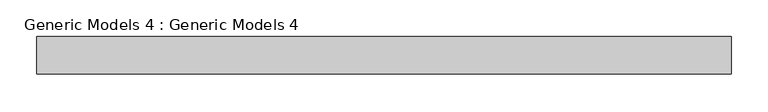
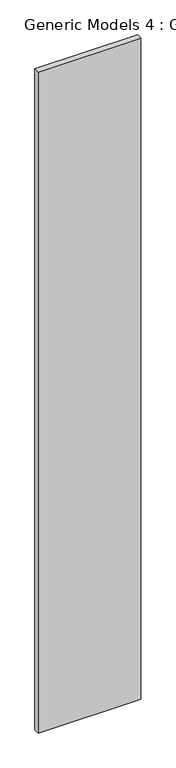
"""IFC4 building model written with IfcOpenShell, lengths in millimetres: proxy geometry, Generic Models 4 : Generic Models 4."""

from ifc_helpers import new_model, si_unit, origin, origin_with_axes, place, context, project, spatial, polyline, outline, extrude, source, transform, mapped, element, save


def generic_models_4_generic_models_4_e71d7c83(model_context):
    return source(origin(), model_context, "Body", "SweptSolid", [
        extrude(outline(polyline([(-11107.9539306, -7500.7844117), (-12049.6586008, -7500.7844117), (-12049.6586008, -7449.9844117), (-11107.9539306, -7449.9844117), (-11107.9539306, -7500.7844117)])), origin_with_axes(), (0.0, 0.0, 1.0), 6400.8),
    ])


if __name__ == "__main__":
    model = new_model("IFC4")
    model_context = context("Model", 3, world=origin())
    ifc_project = project(units=[si_unit("LENGTHUNIT", "METRE", prefix="MILLI")], contexts=[model_context])
    site = spatial("IfcSite", under=ifc_project)
    building = spatial("IfcBuilding", under=site)
    placement = place(None, origin())
    generic_models_4_generic_models_4_shape = generic_models_4_generic_models_4_e71d7c83(model_context)
    element("IfcBuildingElementProxy", 1, Name="Generic Models 4 : Generic Models 4", ObjectType="Generic Models 4 : Generic Models 4", at=placement, inside=building, context=model_context, shape_type="MappedRepresentation", body=[
        mapped(generic_models_4_generic_models_4_shape, transform((0.0, 0.0, 0.0), x_axis=(1.0, 0.0, 0.0), y_axis=(0.0, 1.0, 0.0), z_axis=(0.0, 0.0, 1.0))),
    ])
    save(model, "model.ifc")

# Revit data of these elements
# Element 1 (IfcBuildingElementProxy, "Generic Models 4 : Generic Models 4")
#   Materials on its faces: "SAND STONE BEIGE CLADDING"
# Materials
#   "SAND STONE BEIGE CLADDING": class "Generic", colour RGB 120 120 120, transparency 0, Cost = 0
